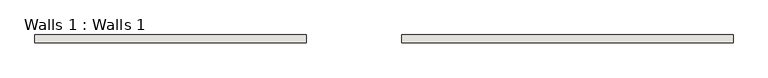
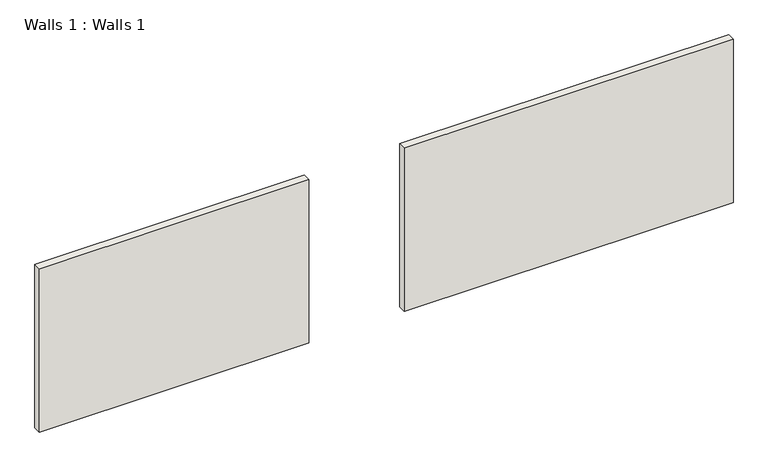
"""IFC4 building model written with IfcOpenShell, lengths in millimetres: wall geometry, Walls 1 : Walls 1."""

from ifc_helpers import new_model, si_unit, origin, origin_with_axes, place, context, project, spatial, polyline, outline, extrude, source, transform, mapped, element, save


def walls_1_walls_1_df8d36ee(model_context):
    return source(origin(), model_context, "Body", "SweptSolid", [
        extrude(outline(polyline([(-2784.6378119, -100.1737531), (-7539.1878119, -100.1737531), (-7539.1878119, 38.1156744), (-2784.6378119, 38.1156744), (-2784.6378119, -100.1737531)])), origin_with_axes(), (0.0, 0.0, 1.0), 3048.0),
        extrude(outline(polyline([(4695.735549, -100.1737531), (-1108.011795, -100.1737531), (-1108.011795, 38.1156744), (4695.735549, 38.1156744), (4695.735549, -100.1737531)])), origin_with_axes(), (0.0, 0.0, 1.0), 3048.0),
    ])


if __name__ == "__main__":
    model = new_model("IFC4")
    model_context = context("Model", 3, world=origin())
    ifc_project = project(units=[si_unit("LENGTHUNIT", "METRE", prefix="MILLI")], contexts=[model_context])
    site = spatial("IfcSite", under=ifc_project)
    building = spatial("IfcBuilding", under=site)
    placement = place(None, origin())
    walls_1_walls_1_shape = walls_1_walls_1_df8d36ee(model_context)
    element("IfcWall", 1, ObjectType="Walls 1 : Walls 1", at=placement, inside=building, context=model_context, shape_type="MappedRepresentation", body=[
        mapped(walls_1_walls_1_shape, transform((0.0, 0.0, 0.0), x_axis=(1.0, 0.0, 0.0), y_axis=(0.0, 1.0, 0.0), z_axis=(0.0, 0.0, 1.0))),
    ])
    save(model, "model.ifc")

# Revit data of these elements
# Element 1 (IfcWall, "Walls 1 : Walls 1")
#   Materials on its faces: "Default Wall"
# Materials
#   "Default Wall": colour RGB 80 80 80, transparency 0
